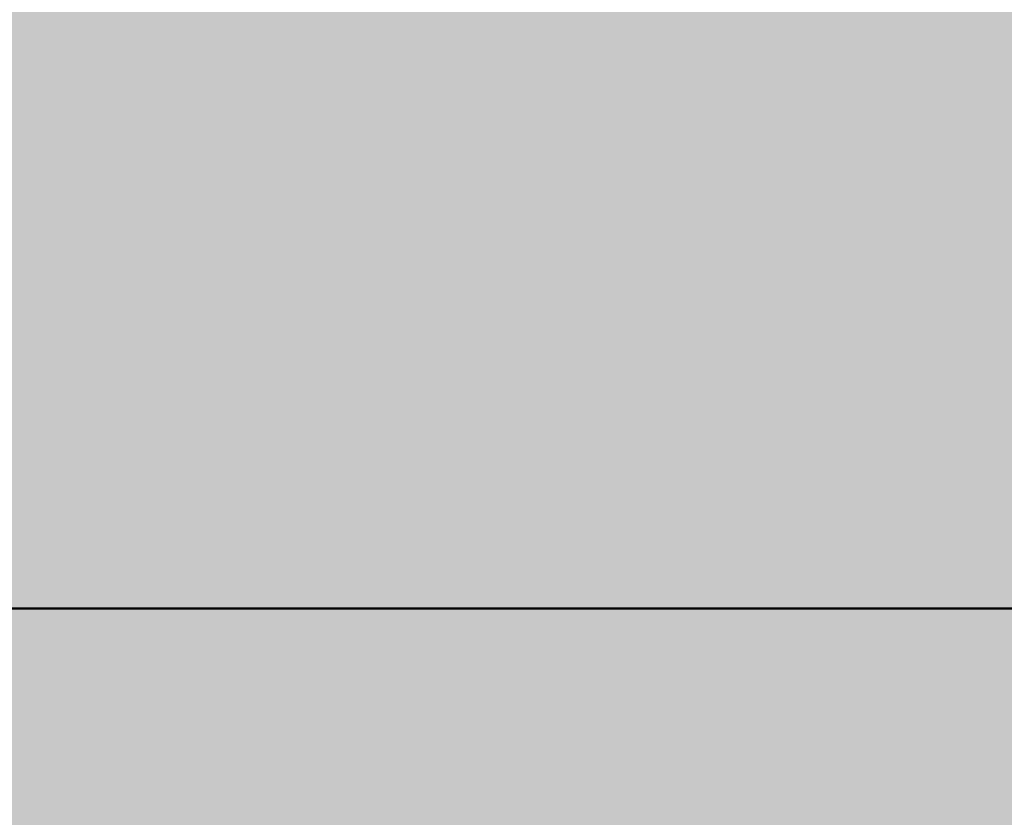
# Model space of a CAD drawing. Units: millimetres. Extents: x 0 to 2267, y 0 to 1823.
# Tile 128 of 256: x 1605.705 to 1611.042, y 1226.115 to 1230.439. Entities that reach past the tile are written whole.
import ezdxf

# ---------------------------------------------------------------- set-up
doc = ezdxf.new("R2010")
doc.units = ezdxf.units.MM
doc.header["$MEASUREMENT"] = 0
doc.layers.add('M-HATC', color=252, linetype='Continuous', lineweight=18)
doc.layers.add('M-OUTL', color=7, linetype='Continuous', lineweight=50)

msp = doc.modelspace()

# ---------------------------------------------------------------- hatches: boundary and pattern name
at = {"layer": 'M-HATC'}
h = msp.add_hatch(color=256, dxfattribs=at)
h.dxf.hatch_style = 1
h.paths.add_polyline_path([(2055.771, 1603.062), (1381.0868, 1603.062), (1381.0868, 1598.062), (2055.771, 1598.062)])
h.paths.add_polyline_path([(2055.771, 1598.062), (1381.0868, 1598.062), (1381.0868, 1593.062), (2055.771, 1593.062)])
h.paths.add_polyline_path([(2051.3074, 1536.7609), (1385.5504, 1536.7609), (1385.5504, 1526.7609), (1387.5504, 1526.7609), (1388.5366, 1525.0528), (1385.3319, 1521.2335), (1385.3319, 1521.2226), (2050.2542, 1522.7491), (2048.3212, 1525.0528), (2049.3074, 1526.7609), (2051.3074, 1526.7609)])
edge = h.paths.add_edge_path()
edge.add_arc((1847.5345, 1379.1492), 135, 222.603061, 222.890851, ccw=False)
edge.add_line((1748.1663, 1287.7656), (1683.0921, 1287.7656))
edge.add_arc((1583.7239, 1379.1492), 135, 317.109149, 317.396939, ccw=False)
edge.add_arc((1678.9686, 1290.6707), 5, 222.8909, 317.1091, ccw=False)
edge.add_arc((1774.2133, 1379.1492), 135, 222.603061, 222.890851, ccw=False)
edge.add_line((1674.8451, 1287.7656), (1609.7709, 1287.7656))
edge.add_arc((1510.4027, 1379.1492), 135, 317.109149, 317.396939, ccw=False)
edge.add_arc((1605.6474, 1290.6707), 5, 222.8909, 317.1091, ccw=False)
edge.add_arc((1700.8921, 1379.1492), 135, 222.603061, 222.890851, ccw=False)
edge.add_line((1601.5239, 1287.7656), (1536.4497, 1287.7656))
edge.add_arc((1437.0815, 1379.1492), 135, 317.109149, 317.396939, ccw=False)
edge.add_arc((1532.3262, 1290.6707), 5, 222.8909, 317.1091, ccw=False)
edge.add_arc((1627.5709, 1379.1492), 135, 222.603061, 222.890851, ccw=False)
edge.add_line((1528.2027, 1287.7656), (1505.9289, 1287.7656))
edge.add_spline(control_points=[(1505.9289, 1287.7656), (1504.2622, 1287.7656), (1504.2622, 1282.7656), (1505.9289, 1282.7656)], knot_values=[0, 0, 0, 0, 5, 5, 5, 5], degree=3, periodic=0)
edge.add_line((1505.9289, 1282.7656), (1930.9289, 1282.7656))
edge.add_spline(control_points=[(1930.9289, 1282.7656), (1932.5956, 1282.7656), (1932.5956, 1287.7656), (1930.9289, 1287.7656)], knot_values=[0, 0, 0, 0, 5, 5, 5, 5], degree=3, periodic=0)
edge.add_line((1930.9289, 1287.7656), (1903.0557, 1287.7656))
edge.add_arc((1803.6875, 1379.1492), 135, 317.109149, 317.396939, ccw=False)
edge.add_arc((1898.9322, 1290.6707), 5, 222.8909, 317.1091, ccw=False)
edge.add_arc((1994.1769, 1379.1492), 135, 222.603061, 222.890851, ccw=False)
edge.add_line((1894.8087, 1287.7656), (1829.7345, 1287.7656))
edge.add_arc((1730.3663, 1379.1492), 135, 317.109149, 317.396939, ccw=False)
edge.add_arc((1825.611, 1290.6707), 5, 222.8909, 317.1091, ccw=False)
edge.add_arc((1920.8557, 1379.1492), 135, 222.603061, 222.890851, ccw=False)
edge.add_line((1821.4875, 1287.7656), (1756.4133, 1287.7656))
edge.add_arc((1657.0451, 1379.1492), 135, 317.109149, 317.396939, ccw=False)
edge.add_arc((1752.2898, 1290.6707), 5, 222.8909, 317.1091, ccw=False)
edge = h.paths.add_edge_path()
edge.add_spline(control_points=[(1843.4289, 1227.2475), (1845.0956, 1227.2475), (1845.0956, 1232.2475), (1843.4289, 1232.2475)], knot_values=[0, 0, 0, 0, 5, 5, 5, 5], degree=3, periodic=0)
edge.add_line((1843.4289, 1232.2475), (1593.4289, 1232.2475))
edge.add_spline(control_points=[(1593.4289, 1232.2475), (1591.7622, 1232.2475), (1591.7622, 1227.2475), (1593.4289, 1227.2475)], knot_values=[0, 0, 0, 0, 5, 5, 5, 5], degree=3, periodic=0)
edge.add_line((1593.4289, 1227.2475), (1843.4289, 1227.2475))
h.paths.add_polyline_path([(1905.9289, 1127.4171), (1530.9289, 1127.4171, 0.414214), (1520.9289, 1117.4171), (1530.9289, 1117.4171), (1915.9289, 1117.4171, 0.414214)])
edge = h.paths.add_edge_path()
edge.add_arc((1397.0858, 1498.4078), 12.7299, 90.78215, 190.87871, ccw=False)
edge.add_line((1396.912, 1511.1365), (1428.0097, 1511.3488))
edge.add_line((1428.0097, 1511.3488), (1433.0097, 1511.3488))
edge.add_line((1433.0097, 1511.3488), (1434.439, 1511.3488))
edge.add_arc((1419.474, 1498.0804), 20, 41.561, 74.08211)
edge.add_line((1424.9592, 1517.3135), (1399.9351, 1517.2561))
edge.add_spline(control_points=[(1399.9307, 1517.2561), (1399.884, 1517.2131), (1399.8328, 1517.1689), (1399.7774, 1517.1236)], knot_values=[11.567499, 11.567499, 11.567499, 11.567499, 11.814249, 11.814249, 11.814249, 11.814249], degree=3, periodic=0)
edge.add_spline(control_points=[(1399.6328, 1517.0099), (1399.5831, 1516.9721), (1399.5307, 1516.9338), (1399.4759, 1516.8947)], knot_values=[11.167718, 11.167718, 11.167718, 11.167718, 11.365188, 11.365188, 11.365188, 11.365188], degree=3, periodic=0)
edge.add_spline(control_points=[(1399.3398, 1516.8001), (1399.1514, 1516.6719), (1398.9384, 1516.5377), (1398.704, 1516.3994)], knot_values=[10.376405, 10.376405, 10.376405, 10.376405, 11.00994, 11.00994, 11.00994, 11.00994], degree=3, periodic=0)
edge.add_spline(control_points=[(1398.6572, 1516.3719), (1398.5789, 1516.326), (1398.4983, 1516.2797), (1398.4155, 1516.2331)], knot_values=[10.125175, 10.125175, 10.125175, 10.125175, 10.334406, 10.334406, 10.334406, 10.334406], degree=3, periodic=0)
edge.add_spline(control_points=[(1398.2642, 1516.1487), (1398.196, 1516.1111), (1398.1263, 1516.0732), (1398.0555, 1516.0351)], knot_values=[9.832246, 9.832246, 9.832246, 9.832246, 9.999658, 9.999658, 9.999658, 9.999658], degree=3, periodic=0)
edge.add_spline(control_points=[(1397.9987, 1516.0048), (1397.7312, 1515.8621), (1397.446, 1515.7171), (1397.1466, 1515.5714)], knot_values=[9.161808, 9.161808, 9.161808, 9.161808, 9.787769, 9.787769, 9.787769, 9.787769], degree=3, periodic=0)
edge.add_spline(control_points=[(1397.1466, 1515.5714), (1396.8418, 1515.423), (1396.5222, 1515.274), (1396.1914, 1515.1262)], knot_values=[8.524455, 8.524455, 8.524455, 8.524455, 9.161808, 9.161808, 9.161808, 9.161808], degree=3, periodic=0)
edge.add_spline(control_points=[(1396.0777, 1515.0756), (1395.9854, 1515.0348), (1395.8922, 1514.994), (1395.7983, 1514.9534)], knot_values=[8.275193, 8.275193, 8.275193, 8.275193, 8.451726, 8.451726, 8.451726, 8.451726], degree=3, periodic=0)
edge.add_spline(control_points=[(1395.6018, 1514.8691), (1395.4997, 1514.8257), (1395.3968, 1514.7824), (1395.2932, 1514.7394)], knot_values=[7.962917, 7.962917, 7.962917, 7.962917, 8.152764, 8.152764, 8.152764, 8.152764], degree=3, periodic=0)
edge.add_spline(control_points=[(1395.2116, 1514.7057), (1394.8278, 1514.5475), (1394.4345, 1514.3929), (1394.0364, 1514.2442)], knot_values=[7.21254, 7.21254, 7.21254, 7.21254, 7.913148, 7.913148, 7.913148, 7.913148], degree=3, periodic=0)
edge.add_spline(control_points=[(1394.0364, 1514.2442), (1393.7076, 1514.1214), (1393.3754, 1514.0027), (1393.0427, 1513.8895)], knot_values=[6.633733, 6.633733, 6.633733, 6.633733, 7.21254, 7.21254, 7.21254, 7.21254], degree=3, periodic=0)
edge.add_spline(control_points=[(1392.8214, 1513.815), (1392.7198, 1513.7812), (1392.6181, 1513.7479), (1392.5166, 1513.7152)], knot_values=[6.328796, 6.328796, 6.328796, 6.328796, 6.505493, 6.505493, 6.505493, 6.505493], degree=3, periodic=0)
edge.add_spline(control_points=[(1392.5166, 1513.7152), (1392.3187, 1513.6515), (1392.1212, 1513.59), (1391.9244, 1513.531)], knot_values=[5.984605, 5.984605, 5.984605, 5.984605, 6.328796, 6.328796, 6.328796, 6.328796], degree=3, periodic=0)
edge.add_spline(control_points=[(1391.7915, 1513.4915), (1391.3122, 1513.3501), (1390.8384, 1513.2239), (1390.3784, 1513.1171)], knot_values=[5.066697, 5.066697, 5.066697, 5.066697, 5.907055, 5.907055, 5.907055, 5.907055], degree=3, periodic=0)
edge.add_spline(control_points=[(1390.3784, 1513.1171), (1390.1797, 1513.071), (1389.9836, 1513.0284), (1389.7907, 1512.9899)], knot_values=[4.70367, 4.70367, 4.70367, 4.70367, 5.066695, 5.066695, 5.066695, 5.066695], degree=3, periodic=0)
edge.add_spline(control_points=[(1389.422, 1512.9204), (1389.2459, 1512.8892), (1389.0729, 1512.8617), (1388.9036, 1512.8381)], knot_values=[4.130571, 4.130571, 4.130571, 4.130571, 4.469816, 4.469816, 4.469816, 4.469816], degree=3, periodic=0)
edge.add_spline(control_points=[(1388.9036, 1512.8381), (1388.591, 1512.7946), (1388.2911, 1512.7644), (1388.0071, 1512.7494)], knot_values=[3.504031, 3.504031, 3.504031, 3.504031, 4.130571, 4.130571, 4.130571, 4.130571], degree=3, periodic=0)
edge.add_spline(control_points=[(1387.9356, 1512.7459), (1387.8538, 1512.7423), (1387.7733, 1512.74), (1387.6944, 1512.739)], knot_values=[3.268866, 3.268866, 3.268866, 3.268866, 3.451164, 3.451164, 3.451164, 3.451164], degree=3, periodic=0)
edge.add_spline(control_points=[(1387.3351, 1512.7443), (1387.2076, 1512.7499), (1387.0847, 1512.7597), (1386.967, 1512.7739)], knot_values=[2.670686, 2.670686, 2.670686, 2.670686, 2.984, 2.984, 2.984, 2.984], degree=3, periodic=0)
edge.add_spline(control_points=[(1386.8327, 1512.7922), (1386.8209, 1512.7941), (1386.8092, 1512.7959), (1386.7975, 1512.7979)], knot_values=[2.516981, 2.516981, 2.516981, 2.516981, 2.549528, 2.549528, 2.549528, 2.549528], degree=3, periodic=0)
edge.add_spline(control_points=[(1386.4526, 1512.8735), (1386.4257, 1512.881), (1386.3993, 1512.889), (1386.3733, 1512.8972)], knot_values=[2.095869, 2.095869, 2.095869, 2.095869, 2.17941, 2.17941, 2.17941, 2.17941], degree=3, periodic=0)
edge.add_spline(control_points=[(1386.0691, 1513.0189), (1386.0634, 1513.0217), (1386.0577, 1513.0246), (1386.052, 1513.0275)], knot_values=[1.72453, 1.72453, 1.72453, 1.72453, 1.745933, 1.745933, 1.745933, 1.745933], degree=3, periodic=0)
edge.add_arc((1399.474, 1498.0804), 20, 131.82432, 180)
edge.add_arc((1630.3336, 1505.5484), 250.9708, 181.705176, 236.427975)
edge.add_arc((1605.3399, 1483.3044), 218.7822, 238.660829, 243.34961)
edge.add_arc((1647.0911, 1510.3592), 262.8986, 183.129836, 237.853442, ccw=False)
h.paths.add_polyline_path([(1406.5369, 1391.9644, 0.149382), (1491.5506, 1296.4418, -0.129517)], flags=17)
edge = h.paths.add_edge_path()
edge.add_arc((2037.3838, 1498.0804), 20, 0, 48.26587)
edge.add_spline(control_points=[(2050.6973, 1513.0052), (2050.6512, 1512.9847), (2050.6034, 1512.9655), (2050.5539, 1512.9477)], knot_values=[1.835652, 1.835652, 1.835652, 1.835652, 2.000781, 2.000781, 2.000781, 2.000781], degree=3, periodic=0)
edge.add_spline(control_points=[(2050.4616, 1512.9166), (2050.479, 1512.9221), (2050.4963, 1512.9277), (2050.5133, 1512.9335)], knot_values=[2.045477, 2.045477, 2.045477, 2.045477, 2.101389, 2.101389, 2.101389, 2.101389], degree=3, periodic=0)
edge.add_spline(control_points=[(2050.129, 1512.8342), (2050.1984, 1512.8473), (2050.2657, 1512.8623), (2050.3308, 1512.8792)], knot_values=[2.237629, 2.237629, 2.237629, 2.237629, 2.435841, 2.435841, 2.435841, 2.435841], degree=3, periodic=0)
edge.add_spline(control_points=[(2050.0946, 1512.8278), (2050.1061, 1512.8299), (2050.1176, 1512.832), (2050.129, 1512.8342)], knot_values=[2.435841, 2.435841, 2.435841, 2.435841, 2.468321, 2.468321, 2.468321, 2.468321], degree=3, periodic=0)
edge.add_spline(control_points=[(2049.7843, 1512.7851), (2049.8552, 1512.7922), (2049.9243, 1512.8008), (2049.9917, 1512.8109)], knot_values=[2.563852, 2.563852, 2.563852, 2.563852, 2.748541, 2.748541, 2.748541, 2.748541], degree=3, periodic=0)
edge.add_spline(control_points=[(2049.4052, 1512.7617), (2049.5364, 1512.7653), (2049.6629, 1512.773), (2049.7843, 1512.7851)], knot_values=[2.748541, 2.748541, 2.748541, 2.748541, 3.064882, 3.064882, 3.064882, 3.064882], degree=3, periodic=0)
edge.add_spline(control_points=[(2049.1698, 1512.7597), (2049.2336, 1512.7591), (2049.2965, 1512.7594), (2049.3584, 1512.7606)], knot_values=[3.102309, 3.102309, 3.102309, 3.102309, 3.2503, 3.2503, 3.2503, 3.2503], degree=3, periodic=0)
edge.add_spline(control_points=[(2048.8573, 1512.7691), (2048.9638, 1512.7638), (2049.068, 1512.7606), (2049.1698, 1512.7597)], knot_values=[3.2503, 3.2503, 3.2503, 3.2503, 3.486069, 3.486069, 3.486069, 3.486069], degree=3, periodic=0)
edge.add_spline(control_points=[(2048.6924, 1512.7789), (2048.3729, 1512.8009), (2048.0345, 1512.8411), (2047.6817, 1512.897)], knot_values=[3.606429, 3.606429, 3.606429, 3.606429, 4.2989, 4.2989, 4.2989, 4.2989], degree=3, periodic=0)
edge.add_spline(control_points=[(2047.6817, 1512.897), (2047.5458, 1512.9185), (2047.4077, 1512.9424), (2047.2678, 1512.9685)], knot_values=[4.2989, 4.2989, 4.2989, 4.2989, 4.565769, 4.565769, 4.565769, 4.565769], degree=3, periodic=0)
edge.add_spline(control_points=[(2047.2678, 1512.9685), (2047.1449, 1512.9914), (2047.0207, 1513.016), (2046.8951, 1513.0422)], knot_values=[4.565769, 4.565769, 4.565769, 4.565769, 4.799971, 4.799971, 4.799971, 4.799971], degree=3, periodic=0)
edge.add_spline(control_points=[(2046.8951, 1513.0422), (2046.5286, 1513.1188), (2046.1513, 1513.209), (2045.7676, 1513.3107)], knot_values=[4.799971, 4.799971, 4.799971, 4.799971, 5.483718, 5.483718, 5.483718, 5.483718], degree=3, periodic=0)
edge.add_spline(control_points=[(2045.7676, 1513.3107), (2045.3724, 1513.4154), (2044.9704, 1513.5322), (2044.5662, 1513.6588)], knot_values=[5.483718, 5.483718, 5.483718, 5.483718, 6.187866, 6.187866, 6.187866, 6.187866], degree=3, periodic=0)
edge.add_spline(control_points=[(2044.5662, 1513.6588), (2044.4149, 1513.7061), (2044.2633, 1513.7549), (2044.1116, 1513.8048)], knot_values=[6.187866, 6.187866, 6.187866, 6.187866, 6.451551, 6.451551, 6.451551, 6.451551], degree=3, periodic=0)
edge.add_spline(control_points=[(2044.1116, 1513.8048), (2043.9967, 1513.8427), (2043.8817, 1513.8813), (2043.7668, 1513.9205)], knot_values=[6.451551, 6.451551, 6.451551, 6.451551, 6.651434, 6.651434, 6.651434, 6.651434], degree=3, periodic=0)
edge.add_spline(control_points=[(2043.7668, 1513.9205), (2043.3716, 1514.0554), (2042.9774, 1514.1979), (2042.5886, 1514.3458)], knot_values=[6.651434, 6.651434, 6.651434, 6.651434, 7.338879, 7.338879, 7.338879, 7.338879], degree=3, periodic=0)
edge.add_spline(control_points=[(2042.5886, 1514.3458), (2042.1643, 1514.5071), (2041.7465, 1514.6749), (2041.3409, 1514.846)], knot_values=[7.338879, 7.338879, 7.338879, 7.338879, 8.089209, 8.089209, 8.089209, 8.089209], degree=3, periodic=0)
edge.add_spline(control_points=[(2041.3409, 1514.846), (2041.1028, 1514.9465), (2040.869, 1515.0481), (2040.6405, 1515.1502)], knot_values=[8.089209, 8.089209, 8.089209, 8.089209, 8.529587, 8.529587, 8.529587, 8.529587], degree=3, periodic=0)
edge.add_spline(control_points=[(2040.51, 1515.2089), (2040.0824, 1515.4022), (2039.6747, 1515.5971), (2039.295, 1515.7894)], knot_values=[8.613818, 8.613818, 8.613818, 8.613818, 9.44571, 9.44571, 9.44571, 9.44571], degree=3, periodic=0)
edge.add_spline(control_points=[(2039.295, 1515.7894), (2039.0618, 1515.9075), (2038.8391, 1516.0246), (2038.6288, 1516.1398)], knot_values=[9.44571, 9.44571, 9.44571, 9.44571, 9.956404, 9.956404, 9.956404, 9.956404], degree=3, periodic=0)
edge.add_spline(control_points=[(2038.6288, 1516.1398), (2038.5187, 1516.2001), (2038.4121, 1516.2598), (2038.309, 1516.3189)], knot_values=[9.956404, 9.956404, 9.956404, 9.956404, 10.223542, 10.223542, 10.223542, 10.223542], degree=3, periodic=0)
edge.add_spline(control_points=[(2038.309, 1516.3189), (2038.2138, 1516.3735), (2038.1216, 1516.4276), (2038.0328, 1516.481)], knot_values=[10.223542, 10.223542, 10.223542, 10.223542, 10.47051, 10.47051, 10.47051, 10.47051], degree=3, periodic=0)
edge.add_spline(control_points=[(2038.0328, 1516.481), (2037.7855, 1516.6296), (2037.5639, 1516.773), (2037.3722, 1516.909)], knot_values=[10.47051, 10.47051, 10.47051, 10.47051, 11.15767, 11.15767, 11.15767, 11.15767], degree=3, periodic=0)
edge.add_spline(control_points=[(2037.3722, 1516.909), (2037.2789, 1516.9752), (2037.1927, 1517.0396), (2037.1142, 1517.102)], knot_values=[11.15767, 11.15767, 11.15767, 11.15767, 11.49227, 11.49227, 11.49227, 11.49227], degree=3, periodic=0)
edge.add_spline(control_points=[(2036.8564, 1517.3259), (2036.9148, 1517.2692), (2036.9814, 1517.2103), (2037.0557, 1517.1492)], knot_values=[11.577341, 11.577341, 11.577341, 11.577341, 11.91035, 11.91035, 11.91035, 11.91035], degree=3, periodic=0)
edge.add_spline(control_points=[(2036.8074, 1517.3748), (2036.823, 1517.3587), (2036.8393, 1517.3424), (2036.8564, 1517.3259)], knot_values=[11.91035, 11.91035, 11.91035, 11.91035, 12.007402, 12.007402, 12.007402, 12.007402], degree=3, periodic=0)
edge.add_spline(control_points=[(2036.7017, 1517.494), (2036.7104, 1517.483), (2036.7196, 1517.4719), (2036.7291, 1517.4606)], knot_values=[12.184155, 12.184155, 12.184155, 12.184155, 12.255409, 12.255409, 12.255409, 12.255409], degree=3, periodic=0)
edge.add_spline(control_points=[(2036.6159, 1517.6205), (2036.62, 1517.613), (2036.6243, 1517.6055), (2036.6289, 1517.5979)], knot_values=[12.487913, 12.487913, 12.487913, 12.487913, 12.541035, 12.541035, 12.541035, 12.541035], degree=3, periodic=0)
edge.add_spline(control_points=[(2036.5635, 1517.786), (2036.5637, 1517.7794), (2036.5642, 1517.7726), (2036.565, 1517.7658)], knot_values=[12.911761, 12.911761, 12.911761, 12.911761, 12.968286, 12.968286, 12.968286, 12.968286], degree=3, periodic=0)
edge.add_spline(control_points=[(2036.6166, 1517.9304), (2036.6125, 1517.9259), (2036.6086, 1517.9212), (2036.6049, 1517.9165)], knot_values=[13.382527, 13.382527, 13.382527, 13.382527, 13.433791, 13.433791, 13.433791, 13.433791], degree=3, periodic=0)
edge.add_spline(control_points=[(2036.749, 1518.017), (2036.7361, 1518.0116), (2036.7239, 1518.006), (2036.7124, 1518.0002)], knot_values=[13.726299, 13.726299, 13.726299, 13.726299, 13.809928, 13.809928, 13.809928, 13.809928], degree=3, periodic=0)
edge.add_spline(control_points=[(2036.8604, 1518.0528), (2036.8386, 1518.0474), (2036.8181, 1518.0416), (2036.7988, 1518.0353)], knot_values=[13.910887, 13.910887, 13.910887, 13.910887, 14.02153, 14.02153, 14.02153, 14.02153], degree=3, periodic=0)
edge.add_line((2036.9639, 1518.0804), (2032.3838, 1518.0804))
edge.add_line((2032.3838, 1518.0804), (2027.3838, 1518.0804))
edge.add_line((2027.3838, 1518.0804), (2022.3838, 1518.0804))
edge.add_line((2022.3838, 1518.0804), (2017.3838, 1518.0804))
edge.add_arc((2017.3838, 1498.0804), 20, 90, 138.439)
edge.add_line((2002.4188, 1511.3488), (2003.8481, 1511.3488))
edge.add_line((2003.8481, 1511.3488), (2008.8481, 1511.3488))
edge.add_line((2008.8481, 1511.3488), (2039.772, 1511.1377))
edge.add_arc((2039.772, 1498.4078), 12.7299, -10.87871, 90, ccw=False)
edge.add_arc((1789.7668, 1510.3592), 262.8986, 302.146558, 356.870164, ccw=False)
edge.add_arc((1831.5179, 1483.3044), 218.7822, 296.65039, 301.339171)
edge.add_arc((1806.5242, 1505.5484), 250.9708, 303.572025, 358.294824)
h.paths.add_polyline_path([(2030.321, 1391.9644, -0.129517), (1945.3072, 1296.4418, 0.149382)], flags=17)
edge = h.paths.add_edge_path()
edge.add_spline(control_points=[(2037.2464, 1518.0821), (2037.2898, 1518.081), (2037.3355, 1518.0804), (2037.3838, 1518.0804)], knot_values=[0.000012, 0.000012, 0.000012, 0.000012, 0.144754, 0.144754, 0.144754, 0.144754], degree=3, periodic=0)
edge.add_line((2037.3357, 1518.0804), (2037.0096, 1518.0804))
edge.add_spline(control_points=[(2037.0096, 1518.0804), (2036.9822, 1518.0768), (2036.956, 1518.0727), (2036.9312, 1518.0681)], knot_values=[14.13465, 14.13465, 14.13465, 14.13465, 14.247197, 14.247197, 14.247197, 14.247197], degree=3, periodic=0)
edge.add_spline(control_points=[(2036.9312, 1518.0681), (2036.9276, 1518.0674), (2036.9241, 1518.0667), (2036.9205, 1518.0661)], knot_values=[14.118315, 14.118315, 14.118315, 14.118315, 14.13465, 14.13465, 14.13465, 14.13465], degree=3, periodic=0)
edge.add_spline(control_points=[(2036.9205, 1518.0661), (2036.9118, 1518.0644), (2036.9032, 1518.0626), (2036.8948, 1518.0608)], knot_values=[14.078086, 14.078086, 14.078086, 14.078086, 14.118315, 14.118315, 14.118315, 14.118315], degree=3, periodic=0)
edge.add_spline(control_points=[(2036.8948, 1518.0608), (2036.883, 1518.0583), (2036.8716, 1518.0556), (2036.8604, 1518.0528)], knot_values=[14.02153, 14.02153, 14.02153, 14.02153, 14.078086, 14.078086, 14.078086, 14.078086], degree=3, periodic=0)
edge.add_spline(control_points=[(2036.8604, 1518.0528), (2036.8386, 1518.0474), (2036.8181, 1518.0416), (2036.7988, 1518.0353)], knot_values=[13.910887, 13.910887, 13.910887, 13.910887, 14.02153, 14.02153, 14.02153, 14.02153], degree=3, periodic=0)
edge.add_spline(control_points=[(2036.7988, 1518.0353), (2036.7981, 1518.035), (2036.7974, 1518.0348), (2036.7967, 1518.0346)], knot_values=[13.906906, 13.906906, 13.906906, 13.906906, 13.910887, 13.910887, 13.910887, 13.910887], degree=3, periodic=0)
edge.add_spline(control_points=[(2036.7967, 1518.0346), (2036.7882, 1518.0318), (2036.7799, 1518.0289), (2036.7719, 1518.0259)], knot_values=[13.857826, 13.857826, 13.857826, 13.857826, 13.906906, 13.906906, 13.906906, 13.906906], degree=3, periodic=0)
edge.add_spline(control_points=[(2036.7719, 1518.0259), (2036.764, 1518.023), (2036.7564, 1518.02), (2036.749, 1518.017)], knot_values=[13.809928, 13.809928, 13.809928, 13.809928, 13.857826, 13.857826, 13.857826, 13.857826], degree=3, periodic=0)
edge.add_spline(control_points=[(2036.749, 1518.017), (2036.7361, 1518.0116), (2036.7239, 1518.006), (2036.7124, 1518.0002)], knot_values=[13.726299, 13.726299, 13.726299, 13.726299, 13.809928, 13.809928, 13.809928, 13.809928], degree=3, periodic=0)
edge.add_spline(control_points=[(2036.7124, 1518.0002), (2036.7121, 1518), (2036.7118, 1517.9999), (2036.7115, 1517.9997)], knot_values=[13.723993, 13.723993, 13.723993, 13.723993, 13.726299, 13.726299, 13.726299, 13.726299], degree=3, periodic=0)
edge.add_spline(control_points=[(2036.7115, 1517.9997), (2036.7063, 1517.9971), (2036.7013, 1517.9944), (2036.6965, 1517.9917)], knot_values=[13.686536, 13.686536, 13.686536, 13.686536, 13.723993, 13.723993, 13.723993, 13.723993], degree=3, periodic=0)
edge.add_spline(control_points=[(2036.6965, 1517.9917), (2036.6919, 1517.9891), (2036.6874, 1517.9865), (2036.6831, 1517.9839)], knot_values=[13.651251, 13.651251, 13.651251, 13.651251, 13.686536, 13.686536, 13.686536, 13.686536], degree=3, periodic=0)
edge.add_spline(control_points=[(2036.6831, 1517.9839), (2036.6764, 1517.9798), (2036.67, 1517.9757), (2036.6639, 1517.9714)], knot_values=[13.596804, 13.596804, 13.596804, 13.596804, 13.651251, 13.651251, 13.651251, 13.651251], degree=3, periodic=0)
edge.add_spline(control_points=[(2036.6639, 1517.9714), (2036.6636, 1517.9712), (2036.6633, 1517.9709), (2036.6629, 1517.9707)], knot_values=[13.593956, 13.593956, 13.593956, 13.593956, 13.596804, 13.596804, 13.596804, 13.596804], degree=3, periodic=0)
edge.add_spline(control_points=[(2036.6629, 1517.9707), (2036.6603, 1517.9689), (2036.6577, 1517.967), (2036.6552, 1517.9651)], knot_values=[13.570322, 13.570322, 13.570322, 13.570322, 13.593956, 13.593956, 13.593956, 13.593956], degree=3, periodic=0)
edge.add_spline(control_points=[(2036.6552, 1517.9651), (2036.6525, 1517.9631), (2036.6499, 1517.9611), (2036.6474, 1517.9591)], knot_values=[13.545477, 13.545477, 13.545477, 13.545477, 13.570322, 13.570322, 13.570322, 13.570322], degree=3, periodic=0)
edge.add_spline(control_points=[(2036.6474, 1517.9591), (2036.6472, 1517.9589), (2036.6471, 1517.9588), (2036.6469, 1517.9587)], knot_values=[13.543931, 13.543931, 13.543931, 13.543931, 13.545477, 13.545477, 13.545477, 13.545477], degree=3, periodic=0)
edge.add_spline(control_points=[(2036.6469, 1517.9587), (2036.6412, 1517.9541), (2036.6358, 1517.9494), (2036.6307, 1517.9447)], knot_values=[13.488237, 13.488237, 13.488237, 13.488237, 13.543931, 13.543931, 13.543931, 13.543931], degree=3, periodic=0)
edge.add_spline(control_points=[(2036.6307, 1517.9447), (2036.6282, 1517.9423), (2036.6257, 1517.9399), (2036.6233, 1517.9374)], knot_values=[13.460307, 13.460307, 13.460307, 13.460307, 13.488237, 13.488237, 13.488237, 13.488237], degree=3, periodic=0)
edge.add_spline(control_points=[(2036.6233, 1517.9374), (2036.6215, 1517.9356), (2036.6198, 1517.9338), (2036.6181, 1517.932)], knot_values=[13.439712, 13.439712, 13.439712, 13.439712, 13.460307, 13.460307, 13.460307, 13.460307], degree=3, periodic=0)
edge.add_spline(control_points=[(2036.6181, 1517.932), (2036.6176, 1517.9315), (2036.6171, 1517.9309), (2036.6166, 1517.9304)], knot_values=[13.433791, 13.433791, 13.433791, 13.433791, 13.439712, 13.439712, 13.439712, 13.439712], degree=3, periodic=0)
edge.add_spline(control_points=[(2036.6166, 1517.9304), (2036.6125, 1517.9259), (2036.6086, 1517.9212), (2036.6049, 1517.9165)], knot_values=[13.382527, 13.382527, 13.382527, 13.382527, 13.433791, 13.433791, 13.433791, 13.433791], degree=3, periodic=0)
edge.add_spline(control_points=[(2036.6049, 1517.9165), (2036.6026, 1517.9135), (2036.6004, 1517.9104), (2036.5982, 1517.9074)], knot_values=[13.350017, 13.350017, 13.350017, 13.350017, 13.382527, 13.382527, 13.382527, 13.382527], degree=3, periodic=0)
edge.add_spline(control_points=[(2036.5982, 1517.9074), (2036.5972, 1517.9059), (2036.5962, 1517.9043), (2036.5952, 1517.9028)], knot_values=[13.333922, 13.333922, 13.333922, 13.333922, 13.350017, 13.350017, 13.350017, 13.350017], degree=3, periodic=0)
edge.add_spline(control_points=[(2036.5952, 1517.9028), (2036.5945, 1517.9018), (2036.5939, 1517.9009), (2036.5933, 1517.8999)], knot_values=[13.323828, 13.323828, 13.323828, 13.323828, 13.333922, 13.333922, 13.333922, 13.333922], degree=3, periodic=0)
edge.add_spline(control_points=[(2036.5933, 1517.8999), (2036.5905, 1517.8955), (2036.5879, 1517.8909), (2036.5855, 1517.8864)], knot_values=[13.277545, 13.277545, 13.277545, 13.277545, 13.323828, 13.323828, 13.323828, 13.323828], degree=3, periodic=0)
edge.add_spline(control_points=[(2036.5855, 1517.8864), (2036.5836, 1517.8827), (2036.5817, 1517.8789), (2036.5801, 1517.8751)], knot_values=[13.240119, 13.240119, 13.240119, 13.240119, 13.277545, 13.277545, 13.277545, 13.277545], degree=3, periodic=0)
edge.add_spline(control_points=[(2036.5801, 1517.8751), (2036.5795, 1517.8739), (2036.579, 1517.8727), (2036.5785, 1517.8715)], knot_values=[13.228211, 13.228211, 13.228211, 13.228211, 13.240119, 13.240119, 13.240119, 13.240119], degree=3, periodic=0)
edge.add_spline(control_points=[(2036.5785, 1517.8715), (2036.578, 1517.8702), (2036.5774, 1517.869), (2036.5769, 1517.8677)], knot_values=[13.215717, 13.215717, 13.215717, 13.215717, 13.228211, 13.228211, 13.228211, 13.228211], degree=3, periodic=0)
edge.add_spline(control_points=[(2036.5769, 1517.8677), (2036.5755, 1517.864), (2036.5741, 1517.8603), (2036.5729, 1517.8565)], knot_values=[13.179847, 13.179847, 13.179847, 13.179847, 13.215717, 13.215717, 13.215717, 13.215717], degree=3, periodic=0)
edge.add_spline(control_points=[(2036.5729, 1517.8565), (2036.5713, 1517.8515), (2036.5699, 1517.8464), (2036.5687, 1517.8413)], knot_values=[13.132017, 13.132017, 13.132017, 13.132017, 13.179847, 13.179847, 13.179847, 13.179847], degree=3, periodic=0)
edge.add_spline(control_points=[(2036.5687, 1517.8413), (2036.5684, 1517.8402), (2036.5682, 1517.8392), (2036.568, 1517.8382)], knot_values=[13.122482, 13.122482, 13.122482, 13.122482, 13.132017, 13.132017, 13.132017, 13.132017], degree=3, periodic=0)
edge.add_spline(control_points=[(2036.568, 1517.8382), (2036.5676, 1517.8363), (2036.5672, 1517.8345), (2036.5669, 1517.8327)], knot_values=[13.105592, 13.105592, 13.105592, 13.105592, 13.122482, 13.122482, 13.122482, 13.122482], degree=3, periodic=0)
edge.add_spline(control_points=[(2036.5669, 1517.8327), (2036.5662, 1517.8292), (2036.5657, 1517.8257), (2036.5652, 1517.8222)], knot_values=[13.074063, 13.074063, 13.074063, 13.074063, 13.105592, 13.105592, 13.105592, 13.105592], degree=3, periodic=0)
edge.add_spline(control_points=[(2036.5652, 1517.8222), (2036.5652, 1517.8222), (2036.5652, 1517.8222), (2036.5652, 1517.8222)], knot_values=[13.074043, 13.074043, 13.074043, 13.074043, 13.074063, 13.074063, 13.074063, 13.074063], degree=3, periodic=0)
edge.add_spline(control_points=[(2036.5652, 1517.8222), (2036.5644, 1517.8164), (2036.5639, 1517.8106), (2036.5636, 1517.8046)], knot_values=[13.021884, 13.021884, 13.021884, 13.021884, 13.074043, 13.074043, 13.074043, 13.074043], degree=3, periodic=0)
edge.add_spline(control_points=[(2036.5636, 1517.8046), (2036.5636, 1517.804), (2036.5636, 1517.8034), (2036.5635, 1517.8028)], knot_values=[13.01674, 13.01674, 13.01674, 13.01674, 13.021884, 13.021884, 13.021884, 13.021884], degree=3, periodic=0)
edge.add_spline(control_points=[(2036.5635, 1517.8028), (2036.5634, 1517.8005), (2036.5634, 1517.7982), (2036.5634, 1517.7958)], knot_values=[12.996438, 12.996438, 12.996438, 12.996438, 13.01674, 13.01674, 13.01674, 13.01674], degree=3, periodic=0)
edge.add_spline(control_points=[(2036.5634, 1517.7958), (2036.5633, 1517.7926), (2036.5634, 1517.7893), (2036.5635, 1517.786)], knot_values=[12.968286, 12.968286, 12.968286, 12.968286, 12.996438, 12.996438, 12.996438, 12.996438], degree=3, periodic=0)
edge.add_spline(control_points=[(2036.5635, 1517.786), (2036.5637, 1517.7794), (2036.5642, 1517.7726), (2036.565, 1517.7658)], knot_values=[12.911761, 12.911761, 12.911761, 12.911761, 12.968286, 12.968286, 12.968286, 12.968286], degree=3, periodic=0)
edge.add_spline(control_points=[(2036.565, 1517.7658), (2036.565, 1517.7657), (2036.565, 1517.7656), (2036.565, 1517.7656)], knot_values=[12.911017, 12.911017, 12.911017, 12.911017, 12.911761, 12.911761, 12.911761, 12.911761], degree=3, periodic=0)
edge.add_spline(control_points=[(2036.565, 1517.7656), (2036.5654, 1517.7625), (2036.5658, 1517.7593), (2036.5663, 1517.7562)], knot_values=[12.88528, 12.88528, 12.88528, 12.88528, 12.911017, 12.911017, 12.911017, 12.911017], degree=3, periodic=0)
edge.add_spline(control_points=[(2036.5663, 1517.7562), (2036.5667, 1517.7534), (2036.5672, 1517.7506), (2036.5677, 1517.7478)], knot_values=[12.862519, 12.862519, 12.862519, 12.862519, 12.88528, 12.88528, 12.88528, 12.88528], degree=3, periodic=0)
edge.add_spline(control_points=[(2036.5677, 1517.7478), (2036.5678, 1517.7474), (2036.5679, 1517.7469), (2036.568, 1517.7465)], knot_values=[12.858885, 12.858885, 12.858885, 12.858885, 12.862519, 12.862519, 12.862519, 12.862519], degree=3, periodic=0)
edge.add_spline(control_points=[(2036.568, 1517.7465), (2036.5692, 1517.7399), (2036.5707, 1517.7332), (2036.5724, 1517.7264)], knot_values=[12.8053, 12.8053, 12.8053, 12.8053, 12.858885, 12.858885, 12.858885, 12.858885], degree=3, periodic=0)
edge.add_spline(control_points=[(2036.5724, 1517.7264), (2036.5734, 1517.7226), (2036.5745, 1517.7187), (2036.5756, 1517.7149)], knot_values=[12.775176, 12.775176, 12.775176, 12.775176, 12.8053, 12.8053, 12.8053, 12.8053], degree=3, periodic=0)
edge.add_spline(control_points=[(2036.5756, 1517.7149), (2036.5763, 1517.7125), (2036.577, 1517.7102), (2036.5778, 1517.7078)], knot_values=[12.756759, 12.756759, 12.756759, 12.756759, 12.775176, 12.775176, 12.775176, 12.775176], degree=3, periodic=0)
edge.add_spline(control_points=[(2036.5778, 1517.7078), (2036.5781, 1517.7067), (2036.5784, 1517.7057), (2036.5787, 1517.7047)], knot_values=[12.748742, 12.748742, 12.748742, 12.748742, 12.756759, 12.756759, 12.756759, 12.756759], degree=3, periodic=0)
edge.add_spline(control_points=[(2036.5787, 1517.7047), (2036.5808, 1517.6983), (2036.5831, 1517.6919), (2036.5856, 1517.6854)], knot_values=[12.69959, 12.69959, 12.69959, 12.69959, 12.748742, 12.748742, 12.748742, 12.748742], degree=3, periodic=0)
edge.add_spline(control_points=[(2036.5856, 1517.6854), (2036.5876, 1517.68), (2036.5898, 1517.6746), (2036.5921, 1517.6692)], knot_values=[12.659038, 12.659038, 12.659038, 12.659038, 12.69959, 12.69959, 12.69959, 12.69959], degree=3, periodic=0)
edge.add_spline(control_points=[(2036.5921, 1517.6692), (2036.594, 1517.6648), (2036.5959, 1517.6605), (2036.5979, 1517.6561)], knot_values=[12.626806, 12.626806, 12.626806, 12.626806, 12.659038, 12.659038, 12.659038, 12.659038], degree=3, periodic=0)
edge.add_spline(control_points=[(2036.5979, 1517.6561), (2036.5984, 1517.6551), (2036.5989, 1517.6541), (2036.5993, 1517.6531)], knot_values=[12.619394, 12.619394, 12.619394, 12.619394, 12.626806, 12.626806, 12.626806, 12.626806], degree=3, periodic=0)
edge.add_spline(control_points=[(2036.5993, 1517.6531), (2036.6043, 1517.6424), (2036.6099, 1517.6315), (2036.6159, 1517.6205)], knot_values=[12.541039, 12.541039, 12.541039, 12.541039, 12.619394, 12.619394, 12.619394, 12.619394], degree=3, periodic=0)
edge.add_spline(control_points=[(2036.6159, 1517.6205), (2036.6159, 1517.6205), (2036.6159, 1517.6205), (2036.6159, 1517.6205)], knot_values=[12.541035, 12.541035, 12.541035, 12.541035, 12.541039, 12.541039, 12.541039, 12.541039], degree=3, periodic=0)
edge.add_spline(control_points=[(2036.6159, 1517.6205), (2036.62, 1517.613), (2036.6243, 1517.6055), (2036.6289, 1517.5979)], knot_values=[12.487913, 12.487913, 12.487913, 12.487913, 12.541035, 12.541035, 12.541035, 12.541035], degree=3, periodic=0)
edge.add_spline(control_points=[(2036.6289, 1517.5979), (2036.6326, 1517.5916), (2036.6365, 1517.5853), (2036.6406, 1517.5789)], knot_values=[12.443982, 12.443982, 12.443982, 12.443982, 12.487913, 12.487913, 12.487913, 12.487913], degree=3, periodic=0)
edge.add_spline(control_points=[(2036.6406, 1517.5789), (2036.6414, 1517.5776), (2036.6423, 1517.5763), (2036.6431, 1517.5749)], knot_values=[12.434996, 12.434996, 12.434996, 12.434996, 12.443982, 12.443982, 12.443982, 12.443982], degree=3, periodic=0)
edge.add_spline(control_points=[(2036.6431, 1517.5749), (2036.6531, 1517.5596), (2036.6639, 1517.5439), (2036.6756, 1517.528)], knot_values=[12.329647, 12.329647, 12.329647, 12.329647, 12.434996, 12.434996, 12.434996, 12.434996], degree=3, periodic=0)
edge.add_spline(control_points=[(2036.6756, 1517.528), (2036.6839, 1517.5168), (2036.6925, 1517.5055), (2036.7017, 1517.494)], knot_values=[12.255409, 12.255409, 12.255409, 12.255409, 12.329647, 12.329647, 12.329647, 12.329647], degree=3, periodic=0)
edge.add_spline(control_points=[(2036.7017, 1517.494), (2036.7104, 1517.483), (2036.7196, 1517.4719), (2036.7291, 1517.4606)], knot_values=[12.184155, 12.184155, 12.184155, 12.184155, 12.255409, 12.255409, 12.255409, 12.255409], degree=3, periodic=0)
edge.add_spline(control_points=[(2036.7291, 1517.4606), (2036.7436, 1517.4435), (2036.759, 1517.4262), (2036.7753, 1517.4085)], knot_values=[12.075961, 12.075961, 12.075961, 12.075961, 12.184155, 12.184155, 12.184155, 12.184155], degree=3, periodic=0)
edge.add_spline(control_points=[(2036.7753, 1517.4085), (2036.7763, 1517.4075), (2036.7773, 1517.4064), (2036.7783, 1517.4054)], knot_values=[12.069502, 12.069502, 12.069502, 12.069502, 12.075961, 12.075961, 12.075961, 12.075961], degree=3, periodic=0)
edge.add_spline(control_points=[(2036.7783, 1517.4054), (2036.7877, 1517.3953), (2036.7974, 1517.385), (2036.8074, 1517.3748)], knot_values=[12.007402, 12.007402, 12.007402, 12.007402, 12.069502, 12.069502, 12.069502, 12.069502], degree=3, periodic=0)
edge.add_spline(control_points=[(2036.8074, 1517.3748), (2036.823, 1517.3587), (2036.8393, 1517.3424), (2036.8564, 1517.3259)], knot_values=[11.91035, 11.91035, 11.91035, 11.91035, 12.007402, 12.007402, 12.007402, 12.007402], degree=3, periodic=0)
edge.add_spline(control_points=[(2036.8564, 1517.3259), (2036.9148, 1517.2692), (2036.9814, 1517.2103), (2037.0557, 1517.1492)], knot_values=[11.577341, 11.577341, 11.577341, 11.577341, 11.91035, 11.91035, 11.91035, 11.91035], degree=3, periodic=0)
edge.add_spline(control_points=[(2037.0557, 1517.1492), (2037.0747, 1517.1336), (2037.0942, 1517.1179), (2037.1142, 1517.102)], knot_values=[11.49227, 11.49227, 11.49227, 11.49227, 11.577341, 11.577341, 11.577341, 11.577341], degree=3, periodic=0)
edge.add_spline(control_points=[(2037.1142, 1517.102), (2037.1927, 1517.0396), (2037.2789, 1516.9752), (2037.3722, 1516.909)], knot_values=[11.15767, 11.15767, 11.15767, 11.15767, 11.49227, 11.49227, 11.49227, 11.49227], degree=3, periodic=0)
edge.add_spline(control_points=[(2037.3722, 1516.909), (2037.5639, 1516.773), (2037.7855, 1516.6296), (2038.0328, 1516.481)], knot_values=[10.47051, 10.47051, 10.47051, 10.47051, 11.15767, 11.15767, 11.15767, 11.15767], degree=3, periodic=0)
edge.add_spline(control_points=[(2038.0328, 1516.481), (2038.1216, 1516.4276), (2038.2138, 1516.3735), (2038.309, 1516.3189)], knot_values=[10.223542, 10.223542, 10.223542, 10.223542, 10.47051, 10.47051, 10.47051, 10.47051], degree=3, periodic=0)
edge.add_spline(control_points=[(2038.309, 1516.3189), (2038.4121, 1516.2598), (2038.5187, 1516.2001), (2038.6288, 1516.1398)], knot_values=[9.956404, 9.956404, 9.956404, 9.956404, 10.223542, 10.223542, 10.223542, 10.223542], degree=3, periodic=0)
edge.add_spline(control_points=[(2038.6288, 1516.1398), (2038.8391, 1516.0246), (2039.0618, 1515.9075), (2039.295, 1515.7894)], knot_values=[9.44571, 9.44571, 9.44571, 9.44571, 9.956404, 9.956404, 9.956404, 9.956404], degree=3, periodic=0)
edge.add_spline(control_points=[(2039.295, 1515.7894), (2039.6747, 1515.5971), (2040.0824, 1515.4022), (2040.51, 1515.2089)], knot_values=[8.613818, 8.613818, 8.613818, 8.613818, 9.44571, 9.44571, 9.44571, 9.44571], degree=3, periodic=0)
edge.add_spline(control_points=[(2040.51, 1515.2089), (2040.5533, 1515.1893), (2040.5968, 1515.1697), (2040.6405, 1515.1502)], knot_values=[8.529587, 8.529587, 8.529587, 8.529587, 8.613818, 8.613818, 8.613818, 8.613818], degree=3, periodic=0)
edge.add_spline(control_points=[(2040.6405, 1515.1502), (2040.869, 1515.0481), (2041.1028, 1514.9465), (2041.3409, 1514.846)], knot_values=[8.089209, 8.089209, 8.089209, 8.089209, 8.529587, 8.529587, 8.529587, 8.529587], degree=3, periodic=0)
edge.add_spline(control_points=[(2041.3409, 1514.846), (2041.7465, 1514.6749), (2042.1643, 1514.5071), (2042.5886, 1514.3458)], knot_values=[7.338879, 7.338879, 7.338879, 7.338879, 8.089209, 8.089209, 8.089209, 8.089209], degree=3, periodic=0)
edge.add_spline(control_points=[(2042.5886, 1514.3458), (2042.9774, 1514.1979), (2043.3716, 1514.0554), (2043.7668, 1513.9205)], knot_values=[6.651434, 6.651434, 6.651434, 6.651434, 7.338879, 7.338879, 7.338879, 7.338879], degree=3, periodic=0)
edge.add_spline(control_points=[(2043.7668, 1513.9205), (2043.8817, 1513.8813), (2043.9967, 1513.8427), (2044.1116, 1513.8048)], knot_values=[6.451551, 6.451551, 6.451551, 6.451551, 6.651434, 6.651434, 6.651434, 6.651434], degree=3, periodic=0)
edge.add_spline(control_points=[(2044.1116, 1513.8048), (2044.2633, 1513.7549), (2044.4149, 1513.7061), (2044.5662, 1513.6588)], knot_values=[6.187866, 6.187866, 6.187866, 6.187866, 6.451551, 6.451551, 6.451551, 6.451551], degree=3, periodic=0)
edge.add_spline(control_points=[(2044.5662, 1513.6588), (2044.9704, 1513.5322), (2045.3724, 1513.4154), (2045.7676, 1513.3107)], knot_values=[5.483718, 5.483718, 5.483718, 5.483718, 6.187866, 6.187866, 6.187866, 6.187866], degree=3, periodic=0)
edge.add_spline(control_points=[(2045.7676, 1513.3107), (2046.1513, 1513.209), (2046.5286, 1513.1188), (2046.8951, 1513.0422)], knot_values=[4.799971, 4.799971, 4.799971, 4.799971, 5.483718, 5.483718, 5.483718, 5.483718], degree=3, periodic=0)
edge.add_spline(control_points=[(2046.8951, 1513.0422), (2047.0207, 1513.016), (2047.1449, 1512.9914), (2047.2678, 1512.9685)], knot_values=[4.565769, 4.565769, 4.565769, 4.565769, 4.799971, 4.799971, 4.799971, 4.799971], degree=3, periodic=0)
edge.add_spline(control_points=[(2047.2678, 1512.9685), (2047.4077, 1512.9424), (2047.5458, 1512.9185), (2047.6817, 1512.897)], knot_values=[4.2989, 4.2989, 4.2989, 4.2989, 4.565769, 4.565769, 4.565769, 4.565769], degree=3, periodic=0)
edge.add_spline(control_points=[(2047.6817, 1512.897), (2048.0345, 1512.8411), (2048.3729, 1512.8009), (2048.6924, 1512.7789)], knot_values=[3.606429, 3.606429, 3.606429, 3.606429, 4.2989, 4.2989, 4.2989, 4.2989], degree=3, periodic=0)
edge.add_spline(control_points=[(2048.6924, 1512.7789), (2048.7479, 1512.7751), (2048.8029, 1512.7718), (2048.8573, 1512.7691)], knot_values=[3.486069, 3.486069, 3.486069, 3.486069, 3.606429, 3.606429, 3.606429, 3.606429], degree=3, periodic=0)
edge.add_spline(control_points=[(2048.8573, 1512.7691), (2048.9638, 1512.7638), (2049.068, 1512.7606), (2049.1698, 1512.7597)], knot_values=[3.2503, 3.2503, 3.2503, 3.2503, 3.486069, 3.486069, 3.486069, 3.486069], degree=3, periodic=0)
edge.add_spline(control_points=[(2049.1698, 1512.7597), (2049.2336, 1512.7591), (2049.2965, 1512.7594), (2049.3584, 1512.7606)], knot_values=[3.102309, 3.102309, 3.102309, 3.102309, 3.2503, 3.2503, 3.2503, 3.2503], degree=3, periodic=0)
edge.add_spline(control_points=[(2049.3584, 1512.7606), (2049.3741, 1512.7609), (2049.3897, 1512.7613), (2049.4052, 1512.7617)], knot_values=[3.064882, 3.064882, 3.064882, 3.064882, 3.102309, 3.102309, 3.102309, 3.102309], degree=3, periodic=0)
edge.add_spline(control_points=[(2049.4052, 1512.7617), (2049.5364, 1512.7653), (2049.6629, 1512.773), (2049.7843, 1512.7851)], knot_values=[2.748541, 2.748541, 2.748541, 2.748541, 3.064882, 3.064882, 3.064882, 3.064882], degree=3, periodic=0)
edge.add_spline(control_points=[(2049.7843, 1512.7851), (2049.8552, 1512.7922), (2049.9243, 1512.8008), (2049.9917, 1512.8109)], knot_values=[2.563852, 2.563852, 2.563852, 2.563852, 2.748541, 2.748541, 2.748541, 2.748541], degree=3, periodic=0)
edge.add_spline(control_points=[(2049.9917, 1512.8109), (2050.0265, 1512.8161), (2050.0608, 1512.8218), (2050.0946, 1512.8278)], knot_values=[2.468321, 2.468321, 2.468321, 2.468321, 2.563852, 2.563852, 2.563852, 2.563852], degree=3, periodic=0)
edge.add_spline(control_points=[(2050.0946, 1512.8278), (2050.1061, 1512.8299), (2050.1176, 1512.832), (2050.129, 1512.8342)], knot_values=[2.435841, 2.435841, 2.435841, 2.435841, 2.468321, 2.468321, 2.468321, 2.468321], degree=3, periodic=0)
edge.add_spline(control_points=[(2050.129, 1512.8342), (2050.1984, 1512.8473), (2050.2657, 1512.8623), (2050.3308, 1512.8792)], knot_values=[2.237629, 2.237629, 2.237629, 2.237629, 2.435841, 2.435841, 2.435841, 2.435841], degree=3, periodic=0)
edge.add_spline(control_points=[(2050.3308, 1512.8792), (2050.3754, 1512.8908), (2050.4191, 1512.9032), (2050.4616, 1512.9166)], knot_values=[2.101389, 2.101389, 2.101389, 2.101389, 2.237629, 2.237629, 2.237629, 2.237629], degree=3, periodic=0)
edge.add_spline(control_points=[(2050.4616, 1512.9166), (2050.479, 1512.9221), (2050.4963, 1512.9277), (2050.5133, 1512.9335)], knot_values=[2.045477, 2.045477, 2.045477, 2.045477, 2.101389, 2.101389, 2.101389, 2.101389], degree=3, periodic=0)
edge.add_spline(control_points=[(2050.5133, 1512.9335), (2050.527, 1512.9382), (2050.5405, 1512.9429), (2050.5539, 1512.9477)], knot_values=[2.000781, 2.000781, 2.000781, 2.000781, 2.045477, 2.045477, 2.045477, 2.045477], degree=3, periodic=0)
edge.add_spline(control_points=[(2050.5539, 1512.9477), (2050.6034, 1512.9655), (2050.6512, 1512.9847), (2050.6973, 1513.0052)], knot_values=[1.835652, 1.835652, 1.835652, 1.835652, 2.000781, 2.000781, 2.000781, 2.000781], degree=3, periodic=0)
edge.add_arc((2037.3838, 1498.0804), 20, 48.26587, 90.12993)
edge = h.paths.add_edge_path(flags=16)
edge.add_spline(control_points=[(1386.1389, 1512.9859), (1388.92, 1511.7395), (1398.0387, 1515.5187), (1399.9307, 1517.2561)], knot_values=[1.831046, 1.831046, 1.831046, 1.831046, 11.814249, 11.814249, 11.814249, 11.814249], degree=3, periodic=0)
edge.add_line((1399.9307, 1517.2561), (1393.7435, 1517.2419))
edge.add_arc((1399.474, 1498.0804), 20, 106.6501, 131.8173)
h = msp.add_hatch(color=256, dxfattribs=at)
h.dxf.hatch_style = 1
h.paths.add_polyline_path([(2042.8886, 1580.1796), (2055.771, 1593.062), (1381.0868, 1593.062), (1393.9692, 1580.1796), (1374.086, 1560.2964), (2062.7718, 1560.2964)])
h.paths.add_polyline_path([(1843.4289, 1201.3297), (1843.4289, 1227.2475), (1593.4289, 1227.2475), (1593.4289, 1201.3297, -0.228274), (1574.5989, 1162.2346), (1530.9289, 1127.4171), (1905.9289, 1127.4171), (1862.2589, 1162.2346, -0.228274)])

# ---------------------------------------------------------------- linework, layer by layer
at = {"layer": 'M-OUTL'}
msp.add_line((1593.4289, 1227.2475), (1843.4289, 1227.2475), dxfattribs=at)

doc.saveas('drawing.dxf')
